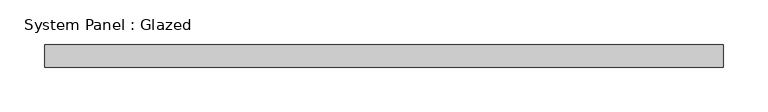
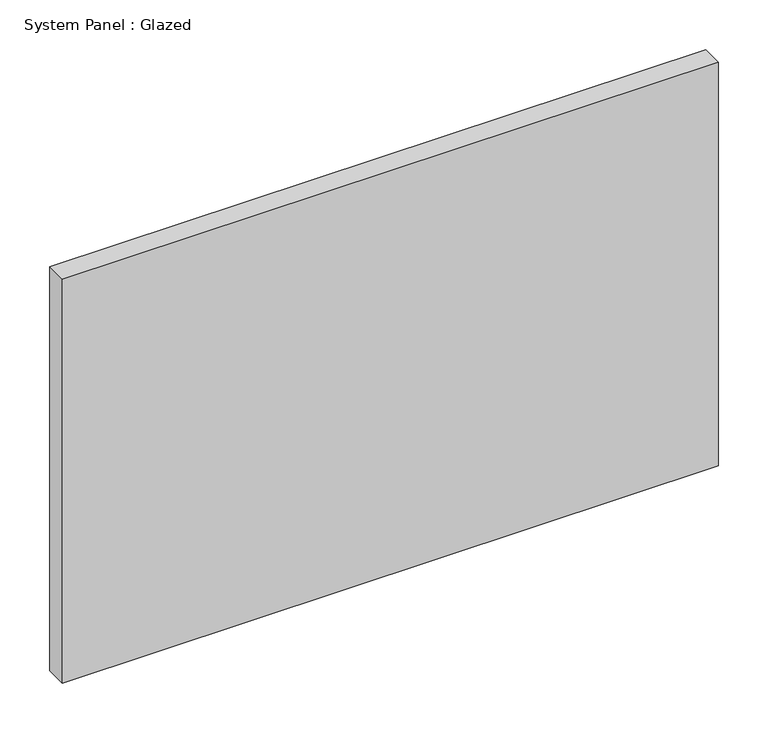
"""IFC4 building model written with IfcOpenShell, lengths in millimetres: plate geometry, System Panel : Glazed."""

from ifc_helpers import new_model, si_unit, origin, origin_with_axes, place, context, project, spatial, polyline, outline, extrude, source, transform, mapped, element, save


def system_panel_glazed_497abead(model_context):
    return source(origin(), model_context, "Body", "SweptSolid", [
        extrude(outline(polyline([(381.0, 19.05), (-381.0, 19.05), (-381.0, 44.45), (381.0, 44.45), (381.0, 19.05)])), origin_with_axes(), (0.0, 0.0, 1.0), 495.6398623),
    ])


if __name__ == "__main__":
    model = new_model("IFC4")
    model_context = context("Model", 3, world=origin())
    ifc_project = project(units=[si_unit("LENGTHUNIT", "METRE", prefix="MILLI")], contexts=[model_context])
    site = spatial("IfcSite", under=ifc_project)
    building = spatial("IfcBuilding", under=site)
    placement = place(None, origin())
    system_panel_glazed_shape = system_panel_glazed_497abead(model_context)
    element("IfcPlate", 1, ObjectType="System Panel : Glazed", at=placement, inside=building, context=model_context, shape_type="MappedRepresentation", body=[
        mapped(system_panel_glazed_shape, transform((0.0, 0.0, 0.0), x_axis=(1.0, 0.0, 0.0), y_axis=(0.0, 1.0, 0.0), z_axis=(0.0, 0.0, 1.0))),
    ])
    save(model, "model.ifc")

# Revit data of these elements
# Type "System Panel : Glazed"
#   Construction Type Id = "GSP4R"
#   Analytic Construction = "1/8 in Pilkington single glazing"
#   Visual Light Transmittance = 0.9
#   Solar Heat Gain Coefficient = 0.86
#   Heat Transfer Coefficient (U) = 1.18115 BTU/(h·ft²·°F)
#   Define Thermal Properties by = 1
# Element 1 (IfcPlate, "System Panel : Glazed")
#   Materials on its faces: "Glass"
# Materials
#   "Glass": class "Glass", colour RGB 0 128 192, transparency 0.75, Description = "Soda Lime Glass", Cost = 0
